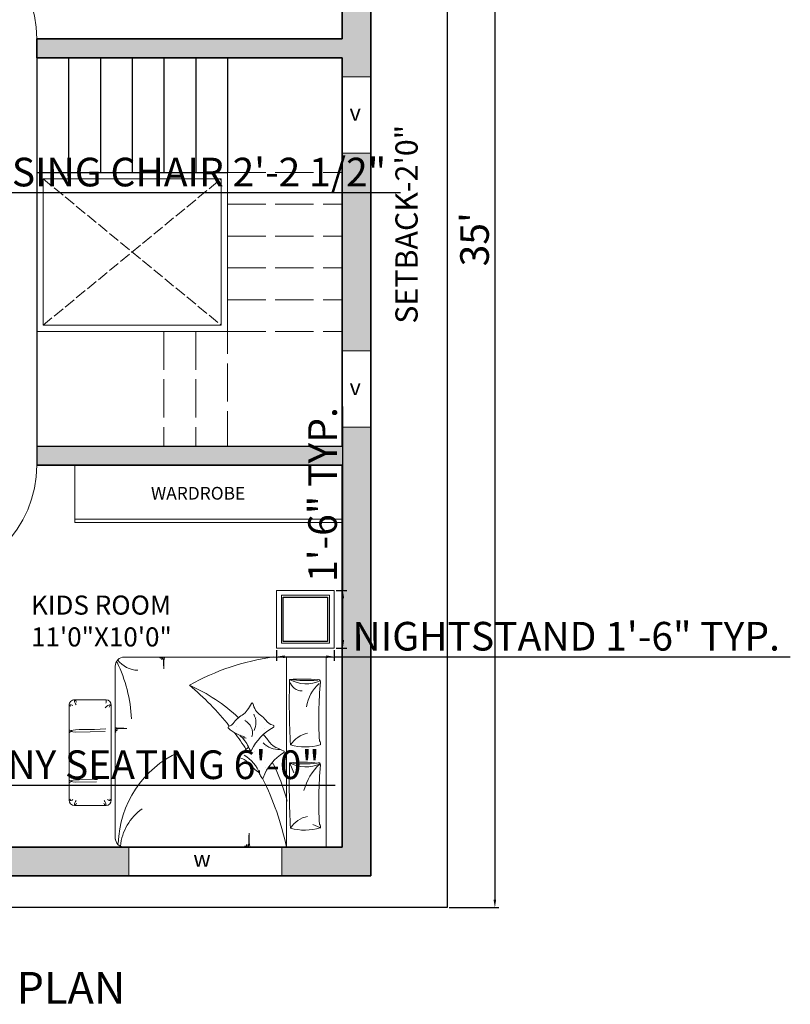
# Model space of a CAD drawing. Units: inches. Extents: x 3488 to 4319, y 780 to 1756.
# Tile 7 of 8: x 4055 to 4298, y 1278 to 1587. Entities that reach past the tile are written whole.
import ezdxf

# ---------------------------------------------------------------- set-up
doc = ezdxf.new("R2010")
doc.units = ezdxf.units.IN
doc.linetypes.add('ACAD_ISO02W100', pattern=[15, 12, -3])
for name, color, linetype, lineweight in [('A-ANNO-IDEN', 7, 'Continuous', 13), ('A-ANNO-TEXT', 7, 'Continuous', 18), ('A-ANNO-TITL', 7, 'Continuous', 25), ('A-AREA-IDEN', 7, 'Continuous', 18), ('A-DOOR', 4, 'Continuous', 18), ('A-FLOR-CASE', 32, 'Continuous', 18), ('A-FLOR-OPEN', 3, 'Continuous', 20), ('A-FLOR-OPEN-HIDN', 3, 'ACAD_ISO02W100', 13), ('A-FLOR-STRS', 7, 'Continuous', 25), ('A-FLOR-STRS-OVHD', 8, 'ACAD_ISO02W100', 18), ('A-WALL', 7, 'Continuous', 35), ('A-WALL-PATT', 252, 'Continuous', 13), ('C-PROP', 7, 'Continuous', 25), ('DIM', 9, 'Continuous', 18), ('FUR', 42, 'Continuous', 18), ('window', 130, 'Continuous', 18)]:
    doc.layers.add(name, color=color, linetype=linetype, lineweight=lineweight)
doc.layers.add('HA-FUR', color=8, linetype='Continuous')
doc.layers.add('wood', color=26, linetype='Continuous')
doc.styles.get("Standard").update_dxf_attribs({"font": 'arial.ttf'})
doc.dimstyles.new('ISO-25', dxfattribs={"dimtxt": 9, "dimasz": 2.5, "dimexe": 1.25, "dimexo": 0.625, "dimtad": 1, "dimdec": 1, "dimlunit": 3, "dimtxsty": 'Standard', "dimcen": 2.5, "dimclrd": 1, "dimclre": 1, "dimclrt": 1, "dimadec": 0, "dimazin": 0, "dimtfac": 1, "dimtdec": 1, "dimtmove": 0, "dimatfit": 3, "dimfxl": 1, "dimarcsym": 0})

# ---------------------------------------------------------------- blocks, each defined once
blk = doc.blocks.new('*U3')
for p, q in [((0, 0), (0, -6)), ((36, 0), (36, -6))]:
    blk.add_line(p, q)
blk.add_lwpolyline([(0, 0), (0, 36), (1.75, 36), (1.75, 0)], close=True)
blk.add_arc((0, 0), 36, 0, 90)
blk = doc.blocks.new('*D8')
at = {"layer": 'Defpoints', "color": 0, "transparency": 16777216}
for p in [(4189.84, 1728.07), (4189.84, 1308.07), (4204.87, 1308.07)]:
    blk.add_point(p, dxfattribs=at)
at = {"layer": 'DIM', "color": 0, "lineweight": -2, "transparency": 16777216}
for p, q in [((4190.47, 1728.07), (4206.12, 1728.07)), ((4204.87, 1725.57), (4204.87, 1310.57)), ((4190.47, 1308.07), (4206.12, 1308.07))]:
    blk.add_line(p, q, dxfattribs=at)
at = {"layer": 'DIM', "color": 0, "transparency": 16777216}
for points in [[(4204.45, 1725.57), (4205.28, 1725.57), (4204.87, 1728.07)], [(4204.45, 1310.57), (4205.28, 1310.57), (4204.87, 1308.07)]]:
    blk.add_solid(points, dxfattribs=at)
at = {"layer": 'DIM', "color": 0, "transparency": 16777216, "insert": (4199.64, 1518.07), "char_height": 9, "attachment_point": 5, "rotation": 90}
blk.add_mtext("35'", dxfattribs=at)
blk = doc.blocks.new('*U9')
for p, q in [((0, 0), (0, 6)), ((36, 0), (36, 6))]:
    blk.add_line(p, q)
blk.add_lwpolyline([(0, 0), (0, -36), (1.75, -36), (1.75, 0)], close=True)
blk.add_arc((0, 0), 36, 270, 0)
blk = doc.blocks.new('*X27')
at = {"color": 0}
for p, q in [((3147.8, 8143.4), (3147.8, 8143.4)), ((3155.9, 8182.9), (3155.9, 8182.9)), ((3209.5, 8023.9), (3209.5, 8023.9)), ((3283, 8049.6), (3283, 8049.6)), ((3154.1, 7950.7), (3154.1, 7950.7)), ((3251.6, 7997), (3251.6, 7997))]:
    blk.add_line(p, q, dxfattribs=at)
blk = doc.blocks.new('*X26')
at = {"color": 0}
for p, q in [((3155.9, 8182.9), (3155.9, 8182.9)), ((3139.8, 7939.7), (3139.8, 7939.7))]:
    blk.add_line(p, q, dxfattribs=at)
blk = doc.blocks.new('*X25')
at = {"color": 0}
for p, q in [((3155.9, 8182.9), (3155.9, 8182.9)), ((3139.8, 7939.7), (3139.8, 7939.7))]:
    blk.add_line(p, q, dxfattribs=at)
blk = doc.blocks.new('*X24')
at = {"color": 0}
for p, q in [((3163, 7776.2), (3163, 7776.2)), ((3422.2, 7761.3), (3422.2, 7761.3)), ((3236.2, 7675.7), (3236.2, 7675.7)), ((3244.3, 7698.6), (3244.3, 7698.6)), ((3340.3, 7689.4), (3340.3, 7689.4))]:
    blk.add_line(p, q, dxfattribs=at)
blk = doc.blocks.new('BED1')
for p, q in [((0, -1000), (0, 800)), ((150, 800), (0, 800)), ((150, 800), (150, -1000)), ((2058.7, 800), (150, 800)), ((528, 800), (528, -1000)), ((211.8, 614.9), (277.5, 585.4)), ((2537.2, 404.9), (2237.2, 404.9)), ((2187.2, 354.9), (2187.2, -545.1)), ((2587.2, -545.1), (2587.2, 354.9)), ((2582, 188.1), (2565.4, 174.8)), ((2566.3, 178.5), (2565.2, 177.4)), ((2565.4, 174.8), (2585.7, 165.4)), ((2566.3, -296.8), (2565.2, -297.9)), ((2582, -287.1), (2565.4, -300.5)), ((2565.4, -300.5), (2585.7, -309.9)), ((2237.2, -595.1), (2537.2, -595.1)), ((150, -1000), (0, -1000)), ((150, -1000), (2063.5, -1000))]:
    blk.add_line(p, q)
for points in [[(934, 797.9), (930.9, 797.7), (928.3, 797.4), (926.3, 796.9), (924.9, 796.3), (923.8, 795.6), (923.1, 794.8), (922.7, 793.8), (922.5, 792.7), (922.4, 791.5), (922.5, 790.3), (922.6, 789.2), (922.6, 788.3), (922.6, 787.6), (922.4, 787.3), (922, 787.4), (921.4, 787.9), (920.6, 788.9), (919.5, 790.2), (918.4, 791.6), (917.1, 793.1), (915.9, 794.6), (914.6, 796), (913.3, 797.1), (912.2, 797.9), (911.1, 798.3), (910.1, 798.4), (909.2, 798), (908.3, 797.1), (907.5, 795.8), (906.8, 793.9), (906, 791.4), (905.4, 788.5), (904.8, 785.2), (904.2, 781.7), (903.7, 778.4), (903.2, 775.4), (902.8, 772.9), (902.5, 771.3), (902.3, 770.6), (902.1, 771.2), (902, 772.8), (901.8, 775.2), (901.7, 778.1), (901.5, 781.5), (901.2, 785), (900.8, 788.4), (900.2, 791.5), (899.5, 794.1), (898.6, 796.2), (897.6, 797.9), (896.5, 799.2), (895.3, 800), (894.1, 800.5), (893, 800.7), (891.9, 800.5), (890.9, 800.1), (890, 799), (889.1, 797.1), (888.3, 794), (887.6, 789.3), (886.9, 782.9), (886.2, 774.2), (885.5, 763.1), (884.8, 749.5), (884.2, 734.2), (883.6, 718.3), (883, 702.8), (882.5, 688.8), (882, 677.5), (881.7, 669.8), (881.5, 666.9), (881.3, 669.4), (881.3, 676.7), (881.3, 687.8), (881.2, 701.5), (881.1, 716.8), (880.8, 732.6), (880.2, 748), (879.4, 761.8), (878.3, 773.2), (876.9, 782.2), (875.1, 789.2), (872.9, 794.4), (870.3, 798), (869, 799)], [(2150, -913.5), (2150, 723.2)], [(494.7, 3.1), (458.9, 95.3)], [(2327.6, 182.3), (2530, 185.9), (2550.8, 181.9), (2561.7, 179), (2566, 176.7), (2566.9, 174.4), (2566.3, 171.9), (2562, 169.2), (2550.3, 166.5), (2527.7, 163.9), (2490.6, 161.8), (2345.5, 160.2), (2317.8, 158.5)], [(2149.7, -259.9), (2150, -268.4), (2150.1, -274.1), (2150.1, -278.1), (2150, -281.4), (2149.8, -284), (2149.5, -286.1), (2149.1, -287.8), (2148.7, -289), (2148.1, -289.9), (2147.4, -290.5), (2146.6, -290.8), (2145.6, -291), (2144.6, -291), (2143.6, -291), (2142.7, -290.9), (2141.9, -290.9), (2141.4, -290.9), (2141.1, -291), (2141.2, -291.4), (2141.7, -291.9), (2142.5, -292.6), (2143.5, -293.4), (2144.7, -294.4), (2146, -295.4), (2147.2, -296.5), (2148.4, -297.6), (2149.3, -298.6), (2150, -299.6), (2150.3, -300.5), (2150.4, -301.3), (2150, -302.1), (2149.3, -302.8), (2148.2, -303.5), (2146.6, -304.1), (2144.6, -304.7), (2142.1, -305.2), (2139.3, -305.7), (2136.5, -306.2), (2133.7, -306.6), (2131.2, -307), (2129.2, -307.3), (2127.8, -307.6), (2127.3, -307.8), (2127.7, -308), (2129, -308.1), (2131, -308.2), (2133.5, -308.3), (2136.3, -308.5), (2139.2, -308.7), (2142, -309), (2144.6, -309.5), (2146.8, -310.1), (2148.6, -310.9), (2150, -311.7), (2151, -312.7), (2151.7, -313.6), (2152.1, -314.6), (2152.3, -315.6), (2152.2, -316.5), (2151.8, -317.3), (2150.9, -318.1), (2149.3, -318.8), (2146.7, -319.4), (2142.8, -320), (2137.4, -320.6), (2130.2, -321.2), (2121, -321.8), (2109.7, -322.3), (2096.9, -322.9), (2083.6, -323.4), (2070.7, -323.9), (2059.1, -324.3), (2049.6, -324.7), (2043.2, -325), (2040.8, -325.2), (2042.9, -325.3), (2049, -325.3), (2058.2, -325.3), (2069.6, -325.4), (2082.3, -325.5), (2095.6, -325.8), (2108.4, -326.2), (2119.9, -326.8), (2129.4, -327.8), (2136.9, -329), (2142.7, -330.5), (2147, -332.3), (2150, -334.4), (2150.9, -335.6)], [(2246.5, -294.4), (2530, -289.4), (2550.8, -293.4), (2561.7, -296.3), (2566, -298.6), (2566.9, -300.8), (2566.3, -303.4), (2562, -306.1), (2550.3, -308.8), (2527.7, -311.3), (2490.6, -313.5), (2345.5, -315), (2238.6, -321.8)], [(1733.7, -998.3), (1731.1, -998.1), (1729, -997.8), (1727.4, -997.4), (1726.1, -997), (1725.2, -996.4), (1724.7, -995.7), (1724.3, -994.8), (1724.1, -993.9), (1724.1, -992.9), (1724.1, -991.9), (1724.2, -991), (1724.2, -990.2), (1724.2, -989.7), (1724.1, -989.4), (1723.8, -989.5), (1723.2, -990), (1722.5, -990.8), (1721.7, -991.8), (1720.7, -993), (1719.7, -994.3), (1718.6, -995.5), (1717.5, -996.6), (1716.5, -997.6), (1715.5, -998.3), (1714.6, -998.6), (1713.8, -998.6), (1713, -998.3), (1712.3, -997.6), (1711.7, -996.5), (1711, -994.9), (1710.4, -992.9), (1709.9, -990.4), (1709.4, -987.6), (1708.9, -984.8), (1708.5, -982), (1708.1, -979.5), (1707.8, -977.4), (1707.5, -976.1), (1707.3, -975.5), (1707.1, -976), (1707, -977.3), (1706.9, -979.3), (1706.8, -981.8), (1706.7, -984.6), (1706.4, -987.5), (1706.1, -990.3), (1705.6, -992.9), (1705, -995.1), (1704.2, -996.9), (1703.4, -998.3), (1702.4, -999.3), (1701.5, -1000), (1700.5, -1000.4), (1699.6, -1000.6), (1698.7, -1000.4), (1697.8, -1000.1), (1697, -999.2), (1696.3, -997.6), (1695.7, -995), (1695.1, -991.1), (1694.5, -985.7), (1693.9, -978.5), (1693.3, -969.3), (1692.8, -957.9), (1692.2, -945.2), (1691.7, -931.9), (1691.2, -919), (1690.8, -907.4), (1690.4, -897.9), (1690.1, -891.5), (1689.9, -889.1), (1689.8, -891.2), (1689.8, -897.3), (1689.8, -906.5), (1689.7, -917.9), (1689.6, -930.6), (1689.4, -943.8), (1688.9, -956.6), (1688.3, -968.1), (1687.3, -977.6), (1686.1, -985.2), (1684.6, -991), (1682.8, -995.3), (1680.7, -998.3), (1679.6, -999.2)]]:
    blk.add_lwpolyline(points)
for points in [[(205.5, 619.6, 0.267769), (215.1, 582.4, -0.037739), (204.3, 21.8, 0.684696), (236.7, 5.5, -0.060702), (497.2, 0.1, -0.046649), (225.9, 3.1, -1.318436)], [(489.2, 619.6, 0.144019), (207.6, 617.9, 0.248643)], [(497.2, 0.1, 0.021276), (489.2, 619.6, -0.206383), (326.6, 509.4, 0.237198)], [(211.8, 12.8, 0.143972), (361.6, 262.9, 1.292232)], [(886.4, -150, -0.069098), (985, -66.5, 0.658965), (982.1, -48.7, -0.049789), (927.4, -29, -0.103757), (896.6, -5.4, 0.055725), (800.9, 83.3, -0.11866), (782.7, 104.9, 0.016811), (761.6, 143.9, 0.70791), (748.3, 144, -0.16964), (551.9, -96.6, 0.664036), (554, -110.7, 0.023706), (627, -144.7, -0.134834), (683.2, -188, 0.012748), (746.3, -267.4)], [(205.5, -168.2, 0.267769), (215.1, -205.4, -0.037739), (204.3, -766, 0.684696), (236.7, -782.3, -0.060702), (497.2, -787.7, -0.046649), (225.9, -784.7, -1.318436)], [(489.2, -168.2, 0.144019), (207.6, -169.9, 0.248643)], [(497.2, -787.7, 0.021276), (489.2, -168.2, -0.206383), (326.6, -278.4, 0.237198)], [(969.1, -259.1, 0.263265), (936.3, -236.9, -0.026108), (909.2, -233.2, 0.027613), (945.1, -234.2, -0.089259), (872.7, -120, 0.662242), (857.6, -119.3, -0.162037), (651.8, -332.7, 0.676499), (654, -354.5, -0.160513), (722.9, -401.5, 0.07473), (773.5, -450.3, -0.187721), (845.5, -559.9, 0.70791), (858.8, -561.4, -0.010003), (898.6, -497.3, -0.113819), (947.3, -450.2, 0.099539), (1032.5, -372.4, -0.173425), (1070.9, -346.4, 0.589988), (1076.2, -326.1, 0.137312), (923.9, -245.9, 0.137312)], [(1446, -733.4, -0.095039), (652.8, -1001.7)]]:
    blk.add_lwpolyline(points, format="xyb")
for centre, radius, start, end in [((3208.8, 1363.3), 2739.4, 191.86791, 206.32469), ((1138.6, 793.9), 983.2, 294.60777, 358.30329), ((1608.1, 842.5), 496.3, 305.19014, 354.02057), ((2062.7, 713.7), 86.5, 0, 93.53765), ((2237.2, 354.9), 50, 90, 180), ((2321.1, 409.7), 84.5, 185.61958, 217.13957), ((2227.5, 373.5), 32.8, 17.83305, 72.80048), ((2546.9, 373.5), 32.8, 107.19952, 162.16695), ((2453.3, 409.7), 84.5, 322.86043, 354.38042), ((2537.2, 354.9), 50, 0, 90), ((2098.7, 754.7), 1625, 193.90497, 207.81692), ((2201.9, 323.3), 34.8, 50.8413, 114.9586), ((2212.2, 381.5), 36.5, 226.80948, 258.3841), ((2572.5, 323.3), 34.8, 65.0414, 129.1587), ((2562.2, 381.5), 36.5, 281.6159, 313.19052), ((751.8, 88.7), 34.9, 336.83517, 27.72181), ((684.2, 86), 100.3, 353.675, 10.88198), ((1074.1, 198.8), 306.1, 197.86019, 241.51221), ((341.4, -277.7), 318.5, 60.71255, 115.00895), ((983.7, -79.5), 20.8, 73.79673, 130.45661), ((978.5, -68.6), 14.3, 39.7097, 85.9506), ((602.5, -324), 198.6, 43.20348, 95.05559), ((3208.8, 1363.3), 2739.4, 212.93136, 216.95099), ((981.1, -281.8), 131.1, 164.0372, 243.45361), ((980, -379), 163.4, 152.61037, 209.36102), ((3208.8, 1363.3), 2739.4, 218.63292, 229.94485), ((2098.7, 754.7), 1625, 226.58872, 246.3156), ((3402.5, -342.9), 1408.5, 182.99169, 205.68187), ((-34.4, -471.2), 376.5, 312.01178, 350.96348), ((2178, -513.5), 33, 286.18268, 338.13858), ((2237.2, -545.1), 50, 180, 270), ((2188.1, -476.2), 73, 269.45125, 322.80265), ((2453.3, -600), 84.5, 5.61958, 37.13957), ((2537.2, -545.1), 50, 270, 0), ((2572.5, -513.6), 34.8, 230.8413, 294.9586), ((2562.2, -571.8), 36.5, 46.80948, 78.3841), ((2271.1, -580.9), 35.8, 148.90546, 197.55407), ((2546.9, -563.8), 32.8, 197.83305, 252.80048), ((375.7, -807.4), 128.2, 17.40732, 88.51286), ((341.4, -1065.5), 318.5, 60.71255, 115.00895), ((1929.1, -1126), 250.5, 37.85533, 88.44053), ((2063.5, -913.5), 86.5, 270, 0)]:
    blk.add_arc(centre, radius, start, end)
for name in ['*X26', '*X25', '*X27', '*X24']:
    blk.add_blockref(name, (-2425.3, -8101.4))
blk = doc.blocks.new('A$C647F3D92')
at = {"layer": 'FUR'}
for points in [[(0.6, 0.6), (0, 0.6), (0, 0), (0.6, 0)], [(0.55, 0.55), (0.05, 0.55), (0.05, 0.05), (0.55, 0.05)]]:
    blk.add_lwpolyline(points, close=True, dxfattribs=at)
at = {"layer": 'HA-FUR'}
blk.add_lwpolyline([(0.53, 0.53), (0.07, 0.53), (0.07, 0.07), (0.53, 0.07)], close=True, dxfattribs=at)
blk = doc.blocks.new('A$C38A85F6B')
at = {"layer": 'wood', "xscale": -1, "rotation": 359.9999999999109}
blk.add_blockref('A$C647F3D92', (0.6, 0), dxfattribs=at)
blk = doc.blocks.new('STAIR-UPPER-RETURN-BEYOND')
for p, q in [((60, 86), (60, 0)), ((60, 86), (96, 86)), ((60, 76), (96, 76)), ((60, 66), (96, 66)), ((60, 56), (96, 56)), ((60, 46), (96, 46)), ((0, 36), (96, 36)), ((40, 36), (40, 0)), ((50, 36), (50, 0))]:
    blk.add_line(p, q)
blk = doc.blocks.new('STAIR-UPPER-ARRIVAL-FLIGHT')
for p, q in [((0, 128), (0, 0)), ((10, 128), (10, 92)), ((20, 128), (20, 92)), ((30, 128), (30, 92)), ((40, 128), (40, 92)), ((50, 128), (50, 92)), ((60, 128), (60, 92)), ((0, 92), (60, 92))]:
    blk.add_line(p, q)
blk = doc.blocks.new('OPENING-STAIRWELL-FRAME')
for points in [[(60, 50), (0, 50), (0, 0), (60, 0)], [(58, 48), (2, 48), (2, 2), (58, 2)]]:
    blk.add_lwpolyline(points, close=True)
blk = doc.blocks.new('*D56')
at = {"layer": 'Defpoints', "color": 0, "transparency": 16777216}
for p in [(4136.25, 1389.61), (4154.36, 1389.61), (4154.36, 1386.89)]:
    blk.add_point(p, dxfattribs=at)
at = {"layer": 'DIM', "color": 1, "lineweight": -2, "transparency": 16777216}
for p, q in [((4136.25, 1388.98), (4136.25, 1385.64)), ((4138.75, 1386.89), (4151.86, 1386.89)), ((4154.36, 1388.98), (4154.36, 1385.64)), ((4154.36, 1386.89), (4297.75, 1386.89))]:
    blk.add_line(p, q, dxfattribs=at)
at = {"layer": 'DIM', "color": 1, "transparency": 16777216}
for points in [[(4138.75, 1387.31), (4138.75, 1386.47), (4136.25, 1386.89)], [(4151.86, 1387.31), (4151.86, 1386.47), (4154.36, 1386.89)]]:
    blk.add_solid(points, dxfattribs=at)
at = {"layer": 'DIM', "color": 1, "transparency": 16777216, "insert": (4227.3, 1392.17), "char_height": 9, "attachment_point": 5}
blk.add_mtext('NIGHTSTAND 1\'-6" TYP.', dxfattribs=at)
blk = doc.blocks.new('*D57')
at = {"layer": 'Defpoints', "color": 0, "transparency": 16777216}
for p in [(4154.36, 1407.72), (4157.07, 1407.72), (4154.36, 1389.61)]:
    blk.add_point(p, dxfattribs=at)
at = {"layer": 'DIM', "color": 1, "lineweight": -2, "transparency": 16777216}
for p, q in [((4157.07, 1407.72), (4157.07, 1465.48)), ((4154.98, 1407.72), (4158.32, 1407.72)), ((4157.07, 1392.11), (4157.07, 1405.22)), ((4154.98, 1389.61), (4158.32, 1389.61))]:
    blk.add_line(p, q, dxfattribs=at)
at = {"layer": 'DIM', "color": 1, "transparency": 16777216}
for points in [[(4156.66, 1405.22), (4157.49, 1405.22), (4157.07, 1407.72)], [(4156.66, 1392.11), (4157.49, 1392.11), (4157.07, 1389.61)]]:
    blk.add_solid(points, dxfattribs=at)
at = {"layer": 'DIM', "color": 1, "transparency": 16777216, "insert": (4151.85, 1437.85), "char_height": 9, "attachment_point": 5, "rotation": 90}
blk.add_mtext('1\'-6" TYP.', dxfattribs=at)
blk = doc.blocks.new('*D98')
at = {"layer": 'Defpoints', "color": 0, "transparency": 16777216}
for p in [(3988.67, 1536.73), (4015.22, 1536.73), (4015.22, 1532.75)]:
    blk.add_point(p, dxfattribs=at)
at = {"layer": 'DIM', "color": 1, "lineweight": -2, "transparency": 16777216}
for p, q in [((3988.67, 1536.1), (3988.67, 1531.5)), ((4015.22, 1536.1), (4015.22, 1531.5)), ((3991.17, 1532.75), (4012.72, 1532.75)), ((4015.22, 1532.75), (4175.19, 1532.75))]:
    blk.add_line(p, q, dxfattribs=at)
at = {"layer": 'DIM', "color": 1, "transparency": 16777216}
for points in [[(3991.17, 1533.16), (3991.17, 1532.33), (3988.67, 1532.75)], [(4012.72, 1533.16), (4012.72, 1532.33), (4015.22, 1532.75)]]:
    blk.add_solid(points, dxfattribs=at)
at = {"layer": 'DIM', "color": 1, "transparency": 16777216, "insert": (4096.46, 1538.02), "char_height": 9, "attachment_point": 5}
blk.add_mtext('DRESSING CHAIR 2\'-2 1/2"', dxfattribs=at)
blk = doc.blocks.new('*D100')
at = {"layer": 'Defpoints', "color": 0, "transparency": 16777216}
for p in [(3933.23, 1357.29), (4005.13, 1357.29), (4005.13, 1346.51)]:
    blk.add_point(p, dxfattribs=at)
at = {"layer": 'DIM', "color": 1, "lineweight": -2, "transparency": 16777216}
for p, q in [((3933.23, 1356.67), (3933.23, 1345.26)), ((4005.13, 1356.67), (4005.13, 1345.26)), ((3935.73, 1346.51), (4002.63, 1346.51)), ((4005.13, 1346.51), (4154.67, 1346.51))]:
    blk.add_line(p, q, dxfattribs=at)
at = {"layer": 'DIM', "color": 1, "transparency": 16777216}
for points in [[(3935.73, 1346.93), (3935.73, 1346.09), (3933.23, 1346.51)], [(4002.63, 1346.93), (4002.63, 1346.09), (4005.13, 1346.51)]]:
    blk.add_solid(points, dxfattribs=at)
at = {"layer": 'DIM', "color": 1, "transparency": 16777216, "insert": (4081.15, 1351.79), "char_height": 9, "attachment_point": 5}
blk.add_mtext('BALCONY SEATING 6\'-0"', dxfattribs=at)

msp = doc.modelspace()

# ---------------------------------------------------------------- hatches: boundary and pattern name
at = {"layer": 'A-WALL-PATT', "transparency": 33554687}
h = msp.add_hatch(color=256, dxfattribs=at)
h.dxf.hatch_style = 1
h.paths.add_polyline_path([(4165.84, 1710.07), (3955.84, 1710.07), (3955.84, 1623.07), (3964.84, 1623.07), (3964.84, 1701.07), (4156.84, 1701.07), (4156.84, 1671.07), (4165.84, 1671.07)])
h.paths.add_polyline_path([(4165.84, 1611.07), (4156.84, 1611.07), (4156.84, 1581.07), (4060.84, 1581.07), (4060.84, 1575.07), (4156.84, 1575.07), (4156.84, 1569.1), (4165.84, 1569.1)])
h.paths.add_polyline_path([(3922.84, 1575.07), (3967.84, 1575.07), (3967.84, 1581.07), (3964.84, 1581.07), (3964.84, 1587.07), (3955.84, 1587.07), (3955.84, 1581.07), (3913.84, 1581.07), (3913.84, 1496.07), (3922.84, 1496.07), (3922.84, 1515.07), (3955.84, 1515.07), (3955.84, 1521.07), (3922.84, 1521.07)])
h.paths.add_polyline_path([(4024.84, 1575.07), (4024.84, 1581.07), (3997.84, 1581.07), (3997.84, 1575.07), (4018.84, 1575.07), (4018.84, 1521.07), (3985.84, 1521.07), (3985.84, 1515.07), (4018.84, 1515.07), (4018.84, 1453.07), (3922.84, 1453.07), (3922.84, 1472.07), (3913.84, 1472.07), (3913.84, 1432.07), (3922.84, 1432.07), (3922.84, 1447.07), (4015.84, 1447.07), (4015.84, 1424.51), (4015.84, 1423.07), (4024.84, 1423.07), (4024.84, 1447.07), (4024.84, 1453.07), (4024.84, 1503.07)])
h.paths.add_polyline_path([(3922.84, 1408.07), (3913.84, 1408.07), (3913.84, 1387.07), (4015.84, 1387.07), (4015.84, 1381.07), (4024.84, 1381.07), (4024.84, 1393.07), (4018.84, 1393.07), (3988.84, 1393.07), (3922.84, 1393.07)])
h.paths.add_polyline_path([(4165.84, 1459.04), (4156.84, 1459.04), (4156.84, 1453.07), (4060.84, 1453.07), (4060.84, 1447.07), (4156.84, 1447.07), (4156.84, 1327.07), (4151.87, 1327.07), (4137.84, 1327.07), (4137.84, 1318.07), (4165.84, 1318.07)])
h.paths.add_polyline_path([(4089.84, 1327.07), (4088.55, 1327.07), (4024.84, 1327.07), (4024.84, 1345.07), (4015.84, 1345.07), (4015.84, 1318.07), (4089.84, 1318.07)])
h.paths.add_polyline_path([(4165.84, 1545.1), (4156.84, 1545.1), (4156.84, 1483.04), (4165.84, 1483.04)])

# ---------------------------------------------------------------- linework, layer by layer
at = {"layer": 'A-FLOR-CASE'}
for p, q in [((4072.84, 1447.07), (4072.84, 1429.07)), ((4072.84, 1430.07), (4156.84, 1430.07)), ((4072.84, 1429.07), (4156.84, 1429.07))]:
    msp.add_line(p, q, dxfattribs=at)
at = {"layer": 'A-FLOR-OPEN-HIDN', "ltscale": 0.3}
for p, q in [((4062.84, 1537.07), (4118.84, 1491.07)), ((4062.84, 1491.07), (4118.84, 1537.07))]:
    msp.add_line(p, q, dxfattribs=at)
at = {"layer": 'A-FLOR-STRS'}
msp.add_line((4060.84, 1453.07), (4156.84, 1453.07), dxfattribs=at)
at = {"layer": 'A-WALL'}
for p, q in [((4165.84, 1710.07), (4165.84, 1318.07)), ((4156.84, 1701.07), (4156.84, 1581.07)), ((4060.84, 1581.07), (4156.84, 1581.07)), ((4060.84, 1581.07), (4060.84, 1575.07)), ((4060.84, 1575.07), (4156.84, 1575.07)), ((4156.84, 1575.07), (4156.84, 1453.07)), ((4060.84, 1447.07), (4156.84, 1447.07)), ((4156.84, 1447.07), (4156.84, 1327.07)), ((4024.84, 1327.07), (4156.84, 1327.07)), ((4015.84, 1318.07), (4165.84, 1318.07))]:
    msp.add_line(p, q, dxfattribs=at)
at = {"layer": 'C-PROP'}
for p, q in [((4189.84, 1728.07), (4189.84, 1308.07)), ((4189.84, 1308.07), (3889.84, 1308.07))]:
    msp.add_line(p, q, dxfattribs=at)
at = {"layer": 'window'}
for p, q in [((4156.84, 1569.1), (4165.84, 1569.1)), ((4156.84, 1545.1), (4165.84, 1545.1)), ((4156.84, 1483.04), (4165.84, 1483.04)), ((4156.84, 1459.04), (4165.84, 1459.04)), ((4089.84, 1327.07), (4089.84, 1318.07)), ((4137.84, 1327.07), (4137.84, 1318.07))]:
    msp.add_line(p, q, dxfattribs=at)

# ---------------------------------------------------------------- block references
at = {"layer": 'A-DOOR'}
for name, p in [('*U3', (4024.84, 1581.07)), ('*U9', (4024.84, 1447.07))]:
    msp.add_blockref(name, p, dxfattribs=at)
at = {"layer": 'A-FLOR-OPEN'}
msp.add_blockref('OPENING-STAIRWELL-FRAME', (4060.85, 1489.07), dxfattribs=at)
at = {"layer": 'A-FLOR-STRS'}
msp.add_blockref('STAIR-UPPER-ARRIVAL-FLIGHT', (4060.84, 1447.07), dxfattribs=at)
at = {"layer": 'A-FLOR-STRS-OVHD'}
msp.add_blockref('STAIR-UPPER-RETURN-BEYOND', (4060.84, 1453.07), dxfattribs=at)
at = {"layer": 'FUR', "xscale": 30.18374333319767, "yscale": 30.18374333319767, "zscale": 30.18374333319767}
msp.add_blockref('A$C38A85F6B', (4136.25, 1389.61), dxfattribs=at)
at = {"layer": 'FUR', "xscale": 0.0331718847221821, "yscale": 0.0331718847221821, "zscale": 0.0331718847221821, "rotation": 180}
msp.add_blockref('BED1', (4156.84, 1353.6), dxfattribs=at)

# ---------------------------------------------------------------- texts
at = {"layer": 'A-ANNO-IDEN'}
for s, p in [('v', (4159.18, 1555.38)), ('v', (4159.18, 1469.13)), ('w', (4110.06, 1320.9))]:
    msp.add_text(s, height=5, dxfattribs=at).set_placement(p)
at = {"layer": 'A-ANNO-TEXT', "insert": (4173.59, 1491.54), "char_height": 7, "attachment_point": 1, "rotation": 90}
msp.add_mtext_dynamic_manual_height_columns('\\pxt7;{SETBACK-2\'0"}', width=83.4163, gutter_width=25, heights=[0], dxfattribs=at)
at = {"layer": 'A-ANNO-TEXT', "insert": (4096.75, 1440.26), "char_height": 4, "attachment_point": 1}
msp.add_mtext_dynamic_manual_height_columns('WARDROBE', width=83.4163, gutter_width=25, heights=[0], dxfattribs=at)
at = {"layer": 'A-ANNO-TITL', "insert": (3968.02, 1287.85), "char_height": 10, "attachment_point": 1}
msp.add_mtext_dynamic_manual_height_columns('FIRST FLOOR PLAN', width=202.5735, gutter_width=25, heights=[0], dxfattribs=at)
at = {"layer": 'A-AREA-IDEN', "insert": (4059.05, 1406.12), "char_height": 6, "attachment_point": 1}
msp.add_mtext_dynamic_manual_height_columns('KIDS ROOM\\P11\'0"X10\'0"', width=83.4163, gutter_width=25, heights=[0], dxfattribs=at)

# ---------------------------------------------------------------- dimensions: what is measured, and where the dimension line sits
at = {"layer": 'DIM'}
dim = msp.add_linear_dim(base=(4204.87, 1308.07), p1=(4189.84, 1728.07), p2=(4189.84, 1308.07), angle=90, dimstyle='ISO-25', override={"dimclrd": 0, "dimclre": 0, "dimclrt": 0}, dxfattribs=at)
dim.commit()
dim.dimension.update_dxf_attribs({"geometry": '*D8', "text_midpoint": (4199.64, 1518.07)})
for base, p1, p2, text, picture, middle in [((4015.2208, 1532.7463), (3988.6746, 1536.7283), (4015.2208, 1536.7283), 'DRESSING CHAIR <>', '*D98', (4096.4573, 1538.0248)), ((4154.36, 1386.89), (4136.25, 1389.61), (4154.36, 1389.61), 'NIGHTSTAND <> TYP.', '*D56', (4227.3, 1392.17)), ((4005.13, 1346.51), (3933.23, 1357.29), (4005.13, 1357.29), 'BALCONY SEATING <>', '*D100', (4081.15, 1351.79))]:
    dim = msp.add_linear_dim(base=base, p1=p1, p2=p2, text=text, dimstyle='ISO-25', override={"dimdec": 1, "dimlfac": 1, "dimrnd": 0, "dimzin": 1, "dimdsep": 46, "dimlunit": 4, "dimfrac": 2}, dxfattribs=at)
    dim.commit()
    dim.dimension.update_dxf_attribs({"geometry": picture, "text_midpoint": middle})
dim = msp.add_linear_dim(base=(4157.07, 1407.72), p1=(4154.36, 1389.61), p2=(4154.36, 1407.72), angle=90, text='<> TYP.', dimstyle='ISO-25', override={"dimdec": 1, "dimlfac": 1, "dimrnd": 0, "dimzin": 1, "dimdsep": 46, "dimlunit": 4, "dimfrac": 2}, dxfattribs=at)
dim.commit()
dim.dimension.update_dxf_attribs({"geometry": '*D57', "text_midpoint": (4151.85, 1437.85)})

doc.saveas('drawing.dxf')
